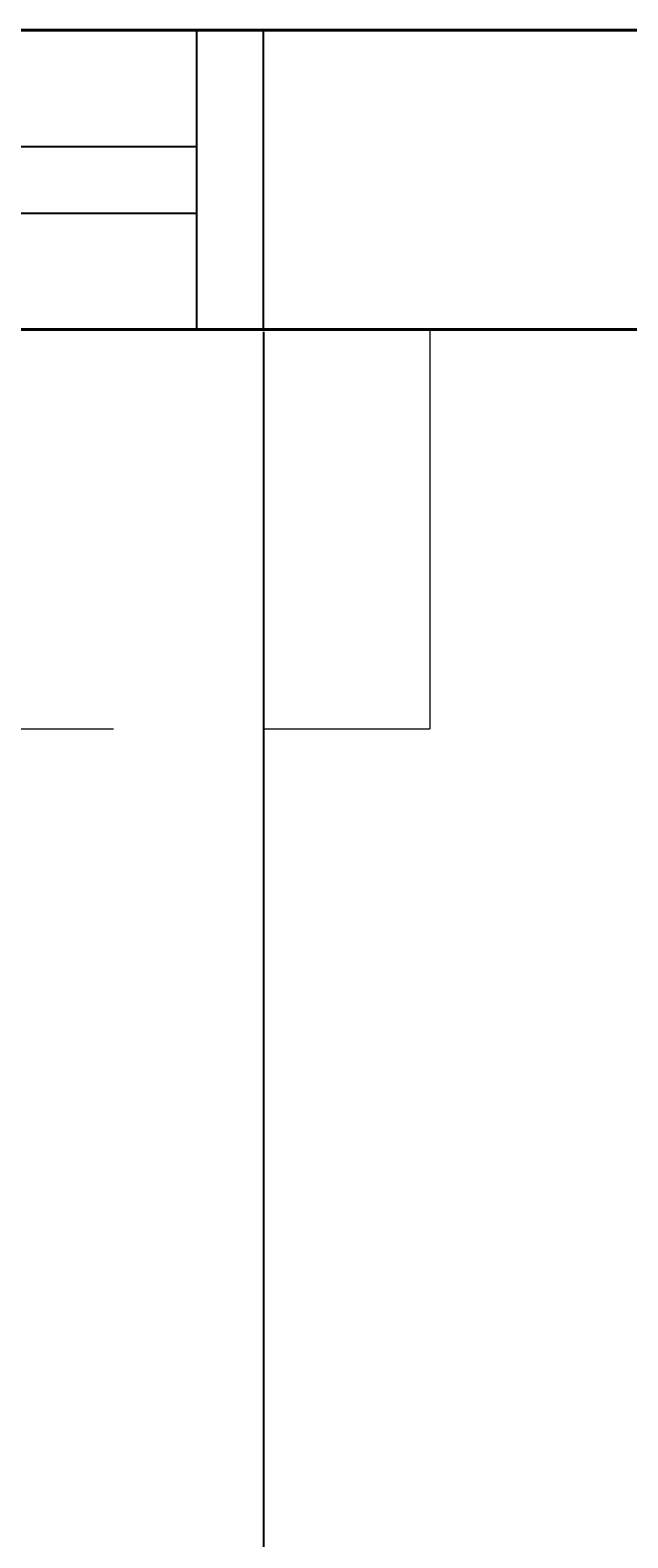
# Model space of a CAD drawing. Units: inches. Extents: x -301 to 715, y -607 to 364.
# Tile 60 of 141: x -111 to -93, y -260 to -215. Entities that reach past the tile are written whole.
import ezdxf

# ---------------------------------------------------------------- set-up
doc = ezdxf.new("R2010")
doc.units = ezdxf.units.IN
doc.header["$MEASUREMENT"] = 0
doc.linetypes.add('ACAD_ISO02W100', pattern=[15, 12, -3])
for name, color, linetype, lineweight in [('A-ANNO-DIMS', 2, 'Continuous', 18), ('A-GLAZ', 2, 'Continuous', 25), ('A-GLAZ-OVHD', 2, 'ACAD_ISO02W100', 18), ('A-WALL', 3, 'Continuous', 40)]:
    doc.layers.add(name, color=color, linetype=linetype, lineweight=lineweight)
doc.styles.get("Standard").update_dxf_attribs({"font": 'arial.ttf'})
doc.dimstyles.get("Standard").update_dxf_attribs({"dimtxt": 0.18, "dimasz": 0.18, "dimexe": 0.18, "dimexo": 0.0625, "dimgap": 0.09, "dimtad": 0, "dimtih": 1, "dimtoh": 1, "dimdec": 1, "dimzin": 0, "dimdsep": 46, "dimlunit": 4, "dimtxsty": 'Standard', "dimcen": 0.09, "dimclrd": 3, "dimclre": 4, "dimclrt": 6, "dimadec": 0, "dimazin": 0, "dimtfac": 1, "dimtdec": 1, "dimtofl": 0, "dimtmove": 0, "dimatfit": 3, "dimfxl": 1, "dimtfill": 2, "dimtfillclr": 51, "dimtolj": 1, "dimtzin": 0, "dimarcsym": 0})

# ---------------------------------------------------------------- blocks, each defined once
blk = doc.blocks.new('WIN-36-PLAN')
for p, q in [((0, 0), (0, 9)), ((2, 0), (2, 9)), ((20, 0), (20, 9)), ((38, 0), (38, 9)), ((40, 0), (40, 9)), ((2, 5.5), (38, 5.5)), ((2, 3.5), (38, 3.5))]:
    blk.add_line(p, q)
blk = doc.blocks.new('WIN-SHADE-50')
at = {"ltscale": 1.5}
for p, q in [((0, 0), (0, 12)), ((50, 12), (0, 12)), ((50, 0), (50, 12)), ((5, 0), (0, 0)), ((45, 0), (50, 0))]:
    blk.add_line(p, q, dxfattribs=at)
blk = doc.blocks.new('*D147')
at = {"layer": 'A-ANNO-DIMS', "color": 4, "lineweight": -2, "transparency": 16777216}
for p, q in [((-103.603, -223.88), (-103.603, -296.865)), ((-45.603, -223.88), (-45.603, -296.865))]:
    blk.add_line(p, q, dxfattribs=at)
at = {"layer": 'A-ANNO-DIMS', "color": 3, "lineweight": -2, "transparency": 16777216}
for p, q in [((-103.423, -296.685), (-75.006, -296.685)), ((-45.783, -296.685), (-74.2, -296.685))]:
    blk.add_line(p, q, dxfattribs=at)
at = {"layer": 'A-ANNO-DIMS', "color": 3, "transparency": 16777216}
for points in [[(-103.423, -296.655), (-103.423, -296.715), (-103.603, -296.685)], [(-45.783, -296.655), (-45.783, -296.715), (-45.603, -296.685)]]:
    blk.add_solid(points, dxfattribs=at)
at = {"layer": 'Defpoints', "color": 0, "transparency": 16777216}
for p in [(-103.603, -223.818), (-45.603, -223.818), (-45.603, -296.685)]:
    blk.add_point(p, dxfattribs=at)
at = {"layer": 'A-ANNO-DIMS', "color": 6, "transparency": 16777216, "insert": (-74.603, -296.685), "char_height": 0.18, "attachment_point": 5, "bg_fill": 1, "box_fill_scale": 1.25, "bg_fill_color": 51, "bg_fill_transparency": 0}
blk.add_mtext('\\A1;4\'-10"', dxfattribs=at)
blk = doc.blocks.new('*D151')
at = {"layer": 'A-ANNO-DIMS', "color": 4, "lineweight": -2, "transparency": 16777216}
for p, q in [((-204.603, -223.755), (-204.603, 359.612)), ((-45.603, -214.755), (-45.603, 359.612))]:
    blk.add_line(p, q, dxfattribs=at)
at = {"layer": 'A-ANNO-DIMS', "color": 3, "lineweight": -2, "transparency": 16777216}
for p, q in [((-204.423, 359.432), (-125.494, 359.432)), ((-45.783, 359.432), (-124.713, 359.432))]:
    blk.add_line(p, q, dxfattribs=at)
at = {"layer": 'A-ANNO-DIMS', "color": 3, "transparency": 16777216}
for points in [[(-204.423, 359.462), (-204.423, 359.402), (-204.603, 359.432)], [(-45.783, 359.462), (-45.783, 359.402), (-45.603, 359.432)]]:
    blk.add_solid(points, dxfattribs=at)
at = {"layer": 'Defpoints', "color": 0, "transparency": 16777216}
for p in [(-45.603, 359.432), (-45.603, -214.818), (-204.603, -223.818)]:
    blk.add_point(p, dxfattribs=at)
at = {"layer": 'A-ANNO-DIMS', "color": 6, "transparency": 16777216, "insert": (-125.103, 359.432), "char_height": 0.18, "attachment_point": 5, "bg_fill": 1, "box_fill_scale": 1.25, "bg_fill_color": 51, "bg_fill_transparency": 0}
blk.add_mtext('\\A1;13\'-3"', dxfattribs=at)
blk = doc.blocks.new('*D158')
at = {"layer": 'A-ANNO-DIMS', "color": 4, "lineweight": -2, "transparency": 16777216}
for p, q in [((-122.603, 221.62), (-122.603, -296.865)), ((-50.603, 221.62), (-50.603, -296.865))]:
    blk.add_line(p, q, dxfattribs=at)
at = {"layer": 'A-ANNO-DIMS', "color": 3, "lineweight": -2, "transparency": 16777216}
for p, q in [((-122.423, -296.685), (-86.933, -296.685)), ((-50.783, -296.685), (-86.274, -296.685))]:
    blk.add_line(p, q, dxfattribs=at)
at = {"layer": 'A-ANNO-DIMS', "color": 3, "transparency": 16777216}
for points in [[(-122.423, -296.655), (-122.423, -296.715), (-122.603, -296.685)], [(-50.783, -296.655), (-50.783, -296.715), (-50.603, -296.685)]]:
    blk.add_solid(points, dxfattribs=at)
at = {"layer": 'Defpoints', "color": 0, "transparency": 16777216}
for p in [(-122.603, 221.682), (-50.603, 221.682), (-50.603, -296.685)]:
    blk.add_point(p, dxfattribs=at)
at = {"layer": 'A-ANNO-DIMS', "color": 6, "transparency": 16777216, "insert": (-86.603, -296.685), "char_height": 0.18, "attachment_point": 5, "bg_fill": 1, "box_fill_scale": 1.25, "bg_fill_color": 51, "bg_fill_transparency": 0}
blk.add_mtext('\\A1;6\'-0"', dxfattribs=at)

msp = doc.modelspace()

# ---------------------------------------------------------------- linework, layer by layer
at = {"layer": 'A-WALL'}
for p, q in [((-195.603, -214.818), (-45.603, -214.818)), ((-204.603, -223.818), (-45.603, -223.818))]:
    msp.add_line(p, q, dxfattribs=at)

# ---------------------------------------------------------------- block references
at = {"layer": 'A-GLAZ'}
msp.add_blockref('WIN-36-PLAN', (-143.603, -223.818), dxfattribs=at)
at = {"layer": 'A-GLAZ-OVHD', "rotation": 180}
msp.add_blockref('WIN-SHADE-50', (-98.604, -223.817), dxfattribs=at)

# ---------------------------------------------------------------- dimensions: what is measured, and where the dimension line sits
at = {"layer": 'A-ANNO-DIMS'}
for base, p1, p2, picture, middle in [((-45.603, 359.432), (-204.603, -223.818), (-45.603, -214.818), '*D151', (-125.103, 359.432)), ((-50.603, -296.685), (-122.603, 221.682), (-50.603, 221.682), '*D158', (-86.603, -296.685)), ((-45.603, -296.685), (-103.603, -223.818), (-45.603, -223.818), '*D147', (-74.603, -296.685))]:
    dim = msp.add_linear_dim(base=base, p1=p1, p2=p2, dimstyle='Standard', override={"dimdec": 1, "dimlfac": 1, "dimrnd": 0, "dimzin": 1, "dimdsep": 46, "dimlunit": 4, "dimfrac": 2}, dxfattribs=at)
    dim.commit()
    dim.dimension.update_dxf_attribs({"geometry": picture, "text_midpoint": middle})

doc.saveas('drawing.dxf')
